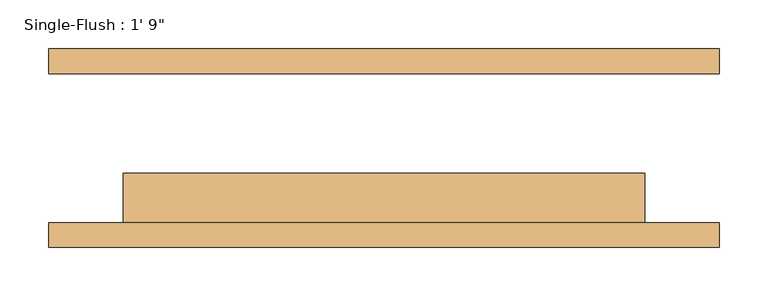
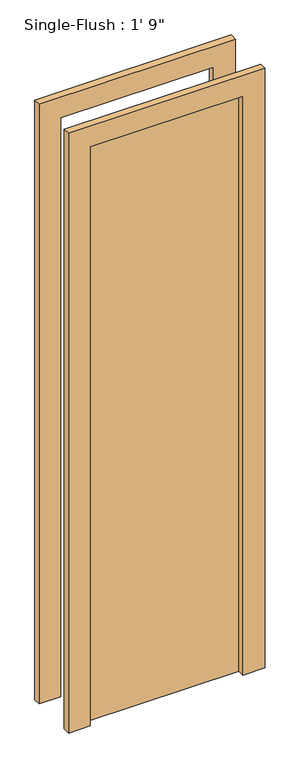
"""IFC4 building model written with IfcOpenShell, lengths in millimetres: door geometry."""

from ifc_helpers import new_model, si_unit, frame, origin, origin_with_axes, place, context, project, spatial, polyline, outline, extrude, source, transform, mapped, element, save


def door_2908be75(model_context):
    return source(origin(), model_context, "Body", "SweptSolid", [
        extrude(outline(polyline([(2209.8, -342.9), (0.0, -342.9), (0.0, -266.7), (2133.6, -266.7), (2133.6, 266.7), (0.0, 266.7), (0.0, 342.9), (2209.8, 342.9), (2209.8, -342.9)])), frame((0.0, -101.6, 0.0), z_axis=(0.0, 1.0, 0.0), x_axis=(0.0, 0.0, 1.0)), (0.0, 0.0, 1.0), 25.4),
        extrude(outline(polyline([(2209.8, 342.9), (2209.8, -342.9), (0.0, -342.9), (0.0, -266.7), (2133.6, -266.7), (2133.6, 266.7), (0.0, 266.7), (0.0, 342.9), (2209.8, 342.9)])), frame((0.0, 76.2, 0.0), z_axis=(0.0, 1.0, 0.0), x_axis=(0.0, 0.0, 1.0)), (0.0, 0.0, 1.0), 25.4),
        extrude(outline(polyline([(266.7, -25.4), (266.7, -76.2), (-266.7, -76.2), (-266.7, -25.4), (266.7, -25.4)])), origin_with_axes(), (0.0, 0.0, 1.0), 2133.6),
    ])


if __name__ == "__main__":
    model = new_model("IFC4")
    model_context = context("Model", 3, world=origin())
    ifc_project = project(units=[si_unit("LENGTHUNIT", "METRE", prefix="MILLI")], contexts=[model_context])
    site = spatial("IfcSite", under=ifc_project)
    building = spatial("IfcBuilding", under=site)
    placement = place(None, origin())
    door_shape = door_2908be75(model_context)
    element("IfcDoor", 1, ObjectType="Single-Flush : 1' 9\"", at=placement, inside=building, context=model_context, shape_type="MappedRepresentation", body=[
        mapped(door_shape, transform((0.0, 0.0, 0.0), x_axis=(1.0, 0.0, 0.0), y_axis=(0.0, 1.0, 0.0), z_axis=(0.0, 0.0, 1.0))),
    ])
    save(model, "model.ifc")

# Revit data of these elements
# Type "Single-Flush : 1' 9\""
#   Type Mark = "10"
#   Construction Type Id = "MDOOR"
#   Assembly Code = "C1020"
#   Analytic Construction = "Metal"
#   Thickness = 0' - 2"
#   Heat Transfer Coefficient (U) = 0.651978 BTU/(h·ft²·°F)
#   Height = 7' - 0"
#   Trim Projection Ext = 0' - 1"
#   Trim Projection Int = 0' - 1"
#   Trim Width = 0' - 3"
#   Width = 1' - 9"
#   Define Thermal Properties by = 1
#   Door Material = Door - Panel
#   Frame Material = Door - Frame
#   Visual Light Transmittance = 0
#   Solar Heat Gain Coefficient = 0
#   Function = (empty or 0)
#   Wall Closure = (empty or 0)
# Element 1 (IfcDoor, "Single-Flush : 1' 9\"")
#   Materials on its faces: "Door - Frame", "Door - Panel"
# Materials
#   "Door - Panel": class "Wood", colour RGB 210 159 95, transparency 0, Cost = 0
#   "Door - Frame": colour RGB 118 70 51, transparency 0, Cost = 0
